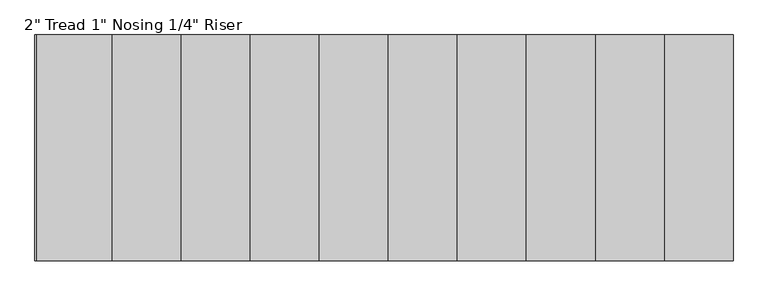
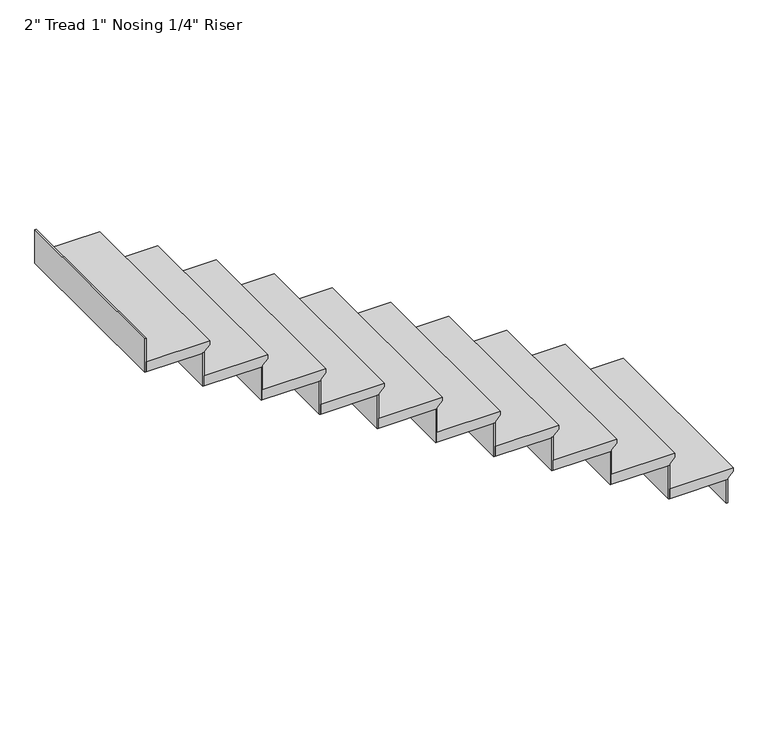
"""IFC4 building model written with IfcOpenShell, lengths in millimetres: stair flight geometry."""

from ifc_helpers import new_model, si_unit, origin, place, context, project, spatial, faceted_brep, source, transform, mapped, element, save


def stair_flight_dce79e7d(model_context):
    return source(origin(), model_context, "Body", "Brep", [
        faceted_brep([(-5990.8517085, 2919.0826226, 3807.8833333), (-5990.8517085, 2919.0826226, 3826.9333333), (-5990.8517085, 2004.6826226, 3826.9333333), (-5990.8517085, 2004.6826226, 3807.8833333), (-6016.2517085, 2919.0826226, 3782.4833333), (-6016.2517085, 2004.6826226, 3782.4833333), (-6295.6517085, 2919.0826226, 3826.9333333), (-6295.6517085, 2004.6826226, 3826.9333333), (-6016.2517085, 2004.6826226, 3776.1333333), (-6295.6517085, 2004.6826226, 3776.1333333), (-6295.6517085, 2919.0826226, 3776.1333333), (-6016.2517085, 2919.0826226, 3776.1333333)], [[[0, 1, 2, 3]], [[4, 0, 3, 5]], [[2, 1, 6, 7]], [[8, 9, 10, 11]], [[2, 7, 9, 8, 5, 3]], [[8, 11, 4, 5]], [[6, 1, 0, 4, 11, 10]], [[7, 6, 10, 9]]]),
        faceted_brep([(-6016.2517085, 2919.0826226, 3776.1333333), (-6016.2517085, 2919.0826226, 3657.6), (-6022.6017085, 2919.0826226, 3657.6), (-6022.6017085, 2919.0826226, 3776.1333333), (-6016.2517085, 2004.6826226, 3776.1333333), (-6022.6017085, 2004.6826226, 3776.1333333), (-6022.6017085, 2004.6826226, 3657.6), (-6016.2517085, 2004.6826226, 3657.6)], [[[0, 1, 2, 3]], [[4, 5, 6, 7]], [[1, 0, 4, 7]], [[2, 1, 7, 6]], [[3, 2, 6, 5]], [[0, 3, 5, 4]]]),
        faceted_brep([(-6295.6517085, 2919.0826226, 3945.4666667), (-6295.6517085, 2919.0826226, 3776.1333333), (-6302.0017085, 2919.0826226, 3776.1333333), (-6302.0017085, 2919.0826226, 3945.4666667), (-6295.6517085, 2004.6826226, 3945.4666667), (-6302.0017085, 2004.6826226, 3945.4666667), (-6302.0017085, 2004.6826226, 3776.1333333), (-6295.6517085, 2004.6826226, 3776.1333333)], [[[0, 1, 2, 3]], [[4, 5, 6, 7]], [[1, 0, 4, 7]], [[2, 1, 7, 6]], [[3, 2, 6, 5]], [[0, 3, 5, 4]]]),
        faceted_brep([(-6270.2517085, 2004.6826226, 3996.2666667), (-6270.2517085, 2919.0826226, 3996.2666667), (-6575.0517085, 2919.0826226, 3996.2666667), (-6575.0517085, 2004.6826226, 3996.2666667), (-6295.6517085, 2004.6826226, 3945.4666667), (-6575.0517085, 2004.6826226, 3945.4666667), (-6575.0517085, 2919.0826226, 3945.4666667), (-6295.6517085, 2919.0826226, 3945.4666667), (-6295.6517085, 2004.6826226, 3951.8166667), (-6270.2517085, 2004.6826226, 3977.2166667), (-6295.6517085, 2919.0826226, 3951.8166667), (-6270.2517085, 2919.0826226, 3977.2166667)], [[[0, 1, 2, 3]], [[4, 5, 6, 7]], [[0, 3, 5, 4, 8, 9]], [[4, 7, 10, 8]], [[2, 1, 11, 10, 7, 6]], [[3, 2, 6, 5]], [[11, 1, 0, 9]], [[10, 11, 9, 8]]]),
        faceted_brep([(-6575.0517085, 2919.0826226, 4114.8), (-6575.0517085, 2919.0826226, 3945.4666667), (-6581.4017085, 2919.0826226, 3945.4666667), (-6581.4017085, 2919.0826226, 4114.8), (-6575.0517085, 2004.6826226, 4114.8), (-6581.4017085, 2004.6826226, 4114.8), (-6581.4017085, 2004.6826226, 3945.4666667), (-6575.0517085, 2004.6826226, 3945.4666667)], [[[0, 1, 2, 3]], [[4, 5, 6, 7]], [[1, 0, 4, 7]], [[2, 1, 7, 6]], [[3, 2, 6, 5]], [[0, 3, 5, 4]]]),
        faceted_brep([(-6549.6517085, 2004.6826226, 4165.6), (-6549.6517085, 2919.0826226, 4165.6), (-6854.4517085, 2919.0826226, 4165.6), (-6854.4517085, 2004.6826226, 4165.6), (-6575.0517085, 2004.6826226, 4114.8), (-6854.4517085, 2004.6826226, 4114.8), (-6854.4517085, 2919.0826226, 4114.8), (-6575.0517085, 2919.0826226, 4114.8), (-6575.0517085, 2004.6826226, 4121.15), (-6549.6517085, 2004.6826226, 4146.55), (-6575.0517085, 2919.0826226, 4121.15), (-6549.6517085, 2919.0826226, 4146.55)], [[[0, 1, 2, 3]], [[4, 5, 6, 7]], [[0, 3, 5, 4, 8, 9]], [[4, 7, 10, 8]], [[2, 1, 11, 10, 7, 6]], [[3, 2, 6, 5]], [[11, 1, 0, 9]], [[10, 11, 9, 8]]]),
        faceted_brep([(-6854.4517085, 2919.0826226, 4284.1333333), (-6854.4517085, 2919.0826226, 4114.8), (-6860.8017085, 2919.0826226, 4114.8), (-6860.8017085, 2919.0826226, 4284.1333333), (-6854.4517085, 2004.6826226, 4284.1333333), (-6860.8017085, 2004.6826226, 4284.1333333), (-6860.8017085, 2004.6826226, 4114.8), (-6854.4517085, 2004.6826226, 4114.8)], [[[0, 1, 2, 3]], [[4, 5, 6, 7]], [[1, 0, 4, 7]], [[2, 1, 7, 6]], [[3, 2, 6, 5]], [[0, 3, 5, 4]]]),
        faceted_brep([(-6829.0517085, 2004.6826226, 4334.9333333), (-6829.0517085, 2919.0826226, 4334.9333333), (-7133.8517085, 2919.0826226, 4334.9333333), (-7133.8517085, 2004.6826226, 4334.9333333), (-6854.4517085, 2004.6826226, 4284.1333333), (-7133.8517085, 2004.6826226, 4284.1333333), (-7133.8517085, 2919.0826226, 4284.1333333), (-6854.4517085, 2919.0826226, 4284.1333333), (-6854.4517085, 2004.6826226, 4290.4833333), (-6829.0517085, 2004.6826226, 4315.8833333), (-6854.4517085, 2919.0826226, 4290.4833333), (-6829.0517085, 2919.0826226, 4315.8833333)], [[[0, 1, 2, 3]], [[4, 5, 6, 7]], [[0, 3, 5, 4, 8, 9]], [[4, 7, 10, 8]], [[2, 1, 11, 10, 7, 6]], [[3, 2, 6, 5]], [[11, 1, 0, 9]], [[10, 11, 9, 8]]]),
        faceted_brep([(-7133.8517085, 2919.0826226, 4453.4666667), (-7133.8517085, 2919.0826226, 4284.1333333), (-7140.2017085, 2919.0826226, 4284.1333333), (-7140.2017085, 2919.0826226, 4453.4666667), (-7133.8517085, 2004.6826226, 4453.4666667), (-7140.2017085, 2004.6826226, 4453.4666667), (-7140.2017085, 2004.6826226, 4284.1333333), (-7133.8517085, 2004.6826226, 4284.1333333)], [[[0, 1, 2, 3]], [[4, 5, 6, 7]], [[1, 0, 4, 7]], [[2, 1, 7, 6]], [[3, 2, 6, 5]], [[0, 3, 5, 4]]]),
        faceted_brep([(-7108.4517085, 2004.6826226, 4504.2666667), (-7108.4517085, 2919.0826226, 4504.2666667), (-7413.2517085, 2919.0826226, 4504.2666667), (-7413.2517085, 2004.6826226, 4504.2666667), (-7133.8517085, 2004.6826226, 4453.4666667), (-7413.2517085, 2004.6826226, 4453.4666667), (-7413.2517085, 2919.0826226, 4453.4666667), (-7133.8517085, 2919.0826226, 4453.4666667), (-7133.8517085, 2004.6826226, 4459.8166667), (-7108.4517085, 2004.6826226, 4485.2166667), (-7133.8517085, 2919.0826226, 4459.8166667), (-7108.4517085, 2919.0826226, 4485.2166667)], [[[0, 1, 2, 3]], [[4, 5, 6, 7]], [[0, 3, 5, 4, 8, 9]], [[4, 7, 10, 8]], [[2, 1, 11, 10, 7, 6]], [[3, 2, 6, 5]], [[11, 1, 0, 9]], [[10, 11, 9, 8]]]),
        faceted_brep([(-7413.2517085, 2919.0826226, 4622.8), (-7413.2517085, 2919.0826226, 4453.4666667), (-7419.6017085, 2919.0826226, 4453.4666667), (-7419.6017085, 2919.0826226, 4622.8), (-7413.2517085, 2004.6826226, 4622.8), (-7419.6017085, 2004.6826226, 4622.8), (-7419.6017085, 2004.6826226, 4453.4666667), (-7413.2517085, 2004.6826226, 4453.4666667)], [[[0, 1, 2, 3]], [[4, 5, 6, 7]], [[1, 0, 4, 7]], [[2, 1, 7, 6]], [[3, 2, 6, 5]], [[0, 3, 5, 4]]]),
        faceted_brep([(-7387.8517085, 2004.6826226, 4673.6), (-7387.8517085, 2919.0826226, 4673.6), (-7692.6517085, 2919.0826226, 4673.6), (-7692.6517085, 2004.6826226, 4673.6), (-7413.2517085, 2004.6826226, 4622.8), (-7692.6517085, 2004.6826226, 4622.8), (-7692.6517085, 2919.0826226, 4622.8), (-7413.2517085, 2919.0826226, 4622.8), (-7413.2517085, 2004.6826226, 4629.15), (-7387.8517085, 2004.6826226, 4654.55), (-7413.2517085, 2919.0826226, 4629.15), (-7387.8517085, 2919.0826226, 4654.55)], [[[0, 1, 2, 3]], [[4, 5, 6, 7]], [[0, 3, 5, 4, 8, 9]], [[4, 7, 10, 8]], [[2, 1, 11, 10, 7, 6]], [[3, 2, 6, 5]], [[11, 1, 0, 9]], [[10, 11, 9, 8]]]),
        faceted_brep([(-7692.6517085, 2919.0826226, 4792.1333333), (-7692.6517085, 2919.0826226, 4622.8), (-7699.0017085, 2919.0826226, 4622.8), (-7699.0017085, 2919.0826226, 4792.1333333), (-7692.6517085, 2004.6826226, 4792.1333333), (-7699.0017085, 2004.6826226, 4792.1333333), (-7699.0017085, 2004.6826226, 4622.8), (-7692.6517085, 2004.6826226, 4622.8)], [[[0, 1, 2, 3]], [[4, 5, 6, 7]], [[1, 0, 4, 7]], [[2, 1, 7, 6]], [[3, 2, 6, 5]], [[0, 3, 5, 4]]]),
        faceted_brep([(-7667.2517085, 2004.6826226, 4842.9333333), (-7667.2517085, 2919.0826226, 4842.9333333), (-7972.0517085, 2919.0826226, 4842.9333333), (-7972.0517085, 2004.6826226, 4842.9333333), (-7692.6517085, 2004.6826226, 4792.1333333), (-7972.0517085, 2004.6826226, 4792.1333333), (-7972.0517085, 2919.0826226, 4792.1333333), (-7692.6517085, 2919.0826226, 4792.1333333), (-7692.6517085, 2004.6826226, 4798.4833333), (-7667.2517085, 2004.6826226, 4823.8833333), (-7692.6517085, 2919.0826226, 4798.4833333), (-7667.2517085, 2919.0826226, 4823.8833333)], [[[0, 1, 2, 3]], [[4, 5, 6, 7]], [[0, 3, 5, 4, 8, 9]], [[4, 7, 10, 8]], [[2, 1, 11, 10, 7, 6]], [[3, 2, 6, 5]], [[11, 1, 0, 9]], [[10, 11, 9, 8]]]),
        faceted_brep([(-7972.0517085, 2919.0826226, 4961.4666667), (-7972.0517085, 2919.0826226, 4792.1333333), (-7978.4017085, 2919.0826226, 4792.1333333), (-7978.4017085, 2919.0826226, 4961.4666667), (-7972.0517085, 2004.6826226, 4961.4666667), (-7978.4017085, 2004.6826226, 4961.4666667), (-7978.4017085, 2004.6826226, 4792.1333333), (-7972.0517085, 2004.6826226, 4792.1333333)], [[[0, 1, 2, 3]], [[4, 5, 6, 7]], [[1, 0, 4, 7]], [[2, 1, 7, 6]], [[3, 2, 6, 5]], [[0, 3, 5, 4]]]),
        faceted_brep([(-7946.6517085, 2004.6826226, 5012.2666667), (-7946.6517085, 2919.0826226, 5012.2666667), (-8251.4517085, 2919.0826226, 5012.2666667), (-8251.4517085, 2004.6826226, 5012.2666667), (-7972.0517085, 2004.6826226, 4961.4666667), (-8251.4517085, 2004.6826226, 4961.4666667), (-8251.4517085, 2919.0826226, 4961.4666667), (-7972.0517085, 2919.0826226, 4961.4666667), (-7972.0517085, 2004.6826226, 4967.8166667), (-7946.6517085, 2004.6826226, 4993.2166667), (-7972.0517085, 2919.0826226, 4967.8166667), (-7946.6517085, 2919.0826226, 4993.2166667)], [[[0, 1, 2, 3]], [[4, 5, 6, 7]], [[0, 3, 5, 4, 8, 9]], [[4, 7, 10, 8]], [[2, 1, 11, 10, 7, 6]], [[3, 2, 6, 5]], [[11, 1, 0, 9]], [[10, 11, 9, 8]]]),
        faceted_brep([(-8251.4517085, 2919.0826226, 5130.8), (-8251.4517085, 2919.0826226, 4961.4666667), (-8257.8017085, 2919.0826226, 4961.4666667), (-8257.8017085, 2919.0826226, 5130.8), (-8251.4517085, 2004.6826226, 5130.8), (-8257.8017085, 2004.6826226, 5130.8), (-8257.8017085, 2004.6826226, 4961.4666667), (-8251.4517085, 2004.6826226, 4961.4666667)], [[[0, 1, 2, 3]], [[4, 5, 6, 7]], [[1, 0, 4, 7]], [[2, 1, 7, 6]], [[3, 2, 6, 5]], [[0, 3, 5, 4]]]),
        faceted_brep([(-8226.0517085, 2004.6826226, 5181.6), (-8226.0517085, 2919.0826226, 5181.6), (-8530.8517085, 2919.0826226, 5181.6), (-8530.8517085, 2004.6826226, 5181.6), (-8251.4517085, 2004.6826226, 5130.8), (-8530.8517085, 2004.6826226, 5130.8), (-8530.8517085, 2919.0826226, 5130.8), (-8251.4517085, 2919.0826226, 5130.8), (-8251.4517085, 2004.6826226, 5137.15), (-8226.0517085, 2004.6826226, 5162.55), (-8251.4517085, 2919.0826226, 5137.15), (-8226.0517085, 2919.0826226, 5162.55)], [[[0, 1, 2, 3]], [[4, 5, 6, 7]], [[0, 3, 5, 4, 8, 9]], [[4, 7, 10, 8]], [[2, 1, 11, 10, 7, 6]], [[3, 2, 6, 5]], [[11, 1, 0, 9]], [[10, 11, 9, 8]]]),
        faceted_brep([(-8810.2517085, 2919.0826226, 5469.4666667), (-8810.2517085, 2919.0826226, 5300.1333333), (-8816.6017085, 2919.0826226, 5300.1333333), (-8816.6017085, 2919.0826226, 5469.4666667), (-8810.2517085, 2004.6826226, 5469.4666667), (-8816.6017085, 2004.6826226, 5469.4666667), (-8816.6017085, 2004.6826226, 5300.1333333), (-8810.2517085, 2004.6826226, 5300.1333333)], [[[0, 1, 2, 3]], [[4, 5, 6, 7]], [[1, 0, 4, 7]], [[2, 1, 7, 6]], [[3, 2, 6, 5]], [[0, 3, 5, 4]]]),
        faceted_brep([(-8530.8517085, 2919.0826226, 5300.1333333), (-8530.8517085, 2919.0826226, 5130.8), (-8537.2017085, 2919.0826226, 5130.8), (-8537.2017085, 2919.0826226, 5300.1333333), (-8530.8517085, 2004.6826226, 5300.1333333), (-8537.2017085, 2004.6826226, 5300.1333333), (-8537.2017085, 2004.6826226, 5130.8), (-8530.8517085, 2004.6826226, 5130.8)], [[[0, 1, 2, 3]], [[4, 5, 6, 7]], [[1, 0, 4, 7]], [[2, 1, 7, 6]], [[3, 2, 6, 5]], [[0, 3, 5, 4]]]),
        faceted_brep([(-8505.4517085, 2004.6826226, 5350.9333333), (-8505.4517085, 2919.0826226, 5350.9333333), (-8784.8517085, 2919.0826226, 5350.9333333), (-8810.2517085, 2919.0826226, 5350.9333333), (-8810.2517085, 2004.6826226, 5350.9333333), (-8530.8517085, 2004.6826226, 5300.1333333), (-8810.2517085, 2004.6826226, 5300.1333333), (-8810.2517085, 2919.0826226, 5300.1333333), (-8784.8517085, 2919.0826226, 5300.1333333), (-8530.8517085, 2919.0826226, 5300.1333333), (-8530.8517085, 2004.6826226, 5306.4833333), (-8505.4517085, 2004.6826226, 5331.8833333), (-8530.8517085, 2919.0826226, 5306.4833333), (-8505.4517085, 2919.0826226, 5331.8833333)], [[[0, 1, 2, 3, 4]], [[5, 6, 7, 8, 9]], [[0, 4, 6, 5, 10, 11]], [[5, 9, 12, 10]], [[2, 1, 13, 12, 9, 8]], [[3, 2, 8, 7]], [[4, 3, 7, 6]], [[13, 1, 0, 11]], [[12, 13, 11, 10]]]),
    ])


if __name__ == "__main__":
    model = new_model("IFC4")
    model_context = context("Model", 3, world=origin())
    ifc_project = project(units=[si_unit("LENGTHUNIT", "METRE", prefix="MILLI")], contexts=[model_context])
    site = spatial("IfcSite", under=ifc_project)
    building = spatial("IfcBuilding", under=site)
    placement = place(None, origin())
    stair_flight_shape = stair_flight_dce79e7d(model_context)
    element("IfcStairFlight", 1, ObjectType="2\" Tread 1\" Nosing 1/4\" Riser", at=placement, inside=building, context=model_context, shape_type="MappedRepresentation", body=[
        mapped(stair_flight_shape, transform((0.0, 0.0, 0.0), x_axis=(1.0, 0.0, 0.0), y_axis=(0.0, 1.0, 0.0), z_axis=(0.0, 0.0, 1.0))),
    ])
    save(model, "model.ifc")
